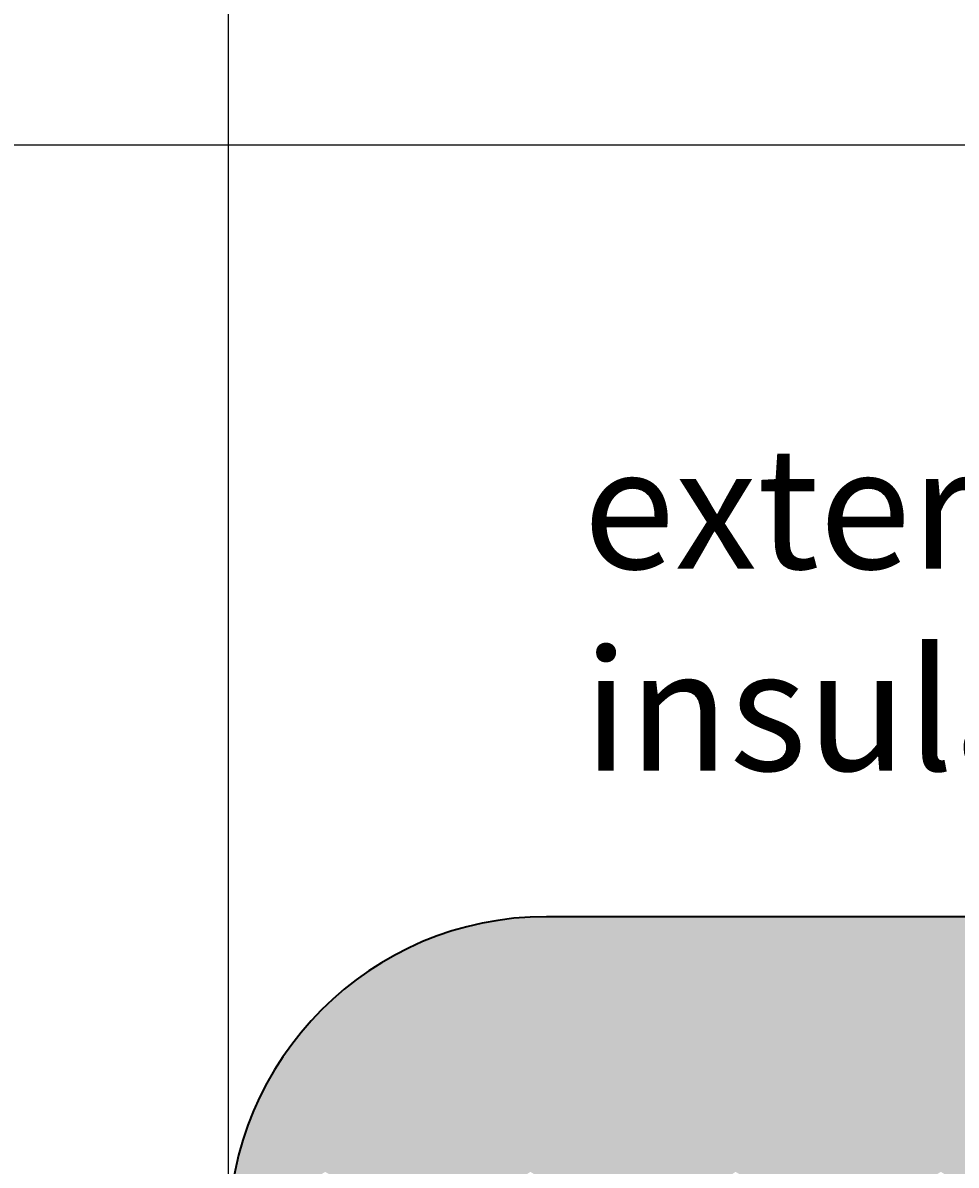
# Model space of a CAD drawing. Units: inches. Extents: x -1 to 292, y -3 to 199.
# Tile 12 of 52: x 45 to 68, y 101 to 130. Entities that reach past the tile are written whole.
import ezdxf

# ---------------------------------------------------------------- set-up
doc = ezdxf.new("R2010")
doc.units = ezdxf.units.IN
doc.header["$MEASUREMENT"] = 0
for name, color, linetype, lineweight in [('M-ANNO-TEXT', 3, 'Continuous', 25), ('M-DIMS', 2, 'Continuous', 18), ('M-EQPM', 7, 'Continuous', 35), ('M-PATT', 8, 'Continuous', 13)]:
    doc.layers.add(name, color=color, linetype=linetype, lineweight=lineweight)
doc.styles.get("Standard").update_dxf_attribs({"font": 'arial.ttf'})
doc.dimstyles.get("Standard").update_dxf_attribs({"dimtxt": 0.18, "dimasz": 0.18, "dimexe": 0.18, "dimexo": 0.0625, "dimgap": 0.09, "dimtad": 0, "dimtih": 1, "dimtoh": 1, "dimdec": 4, "dimzin": 0, "dimdsep": 46, "dimtxsty": 'Standard', "dimcen": 0.09, "dimadec": 0, "dimazin": 0, "dimtfac": 1, "dimtdec": 4, "dimtofl": 0, "dimtmove": 0, "dimatfit": 3, "dimfxl": 1, "dimtolj": 1, "dimtzin": 0, "dimarcsym": 0})

# ---------------------------------------------------------------- blocks, each defined once
blk = doc.blocks.new('*D8')
at = {"layer": 'Defpoints', "color": 0, "transparency": 16777216}
for p in [(-0.662, 126.765), (111.488, 126.765), (69.013, 25.514)]:
    blk.add_point(p, dxfattribs=at)
at = {"layer": 'M-DIMS', "color": 0, "lineweight": -2, "transparency": 16777216}
for p, q in [((111.426, 126.765), (-0.842, 126.765)), ((-0.662, 126.585), (-0.662, 76.321)), ((-0.662, 25.694), (-0.662, 75.958)), ((68.951, 25.514), (-0.842, 25.514))]:
    blk.add_line(p, q, dxfattribs=at)
at = {"layer": 'M-DIMS', "color": 0, "transparency": 16777216}
for points in [[(-0.692, 126.585), (-0.632, 126.585), (-0.662, 126.765)], [(-0.692, 25.694), (-0.632, 25.694), (-0.662, 25.514)]]:
    blk.add_solid(points, dxfattribs=at)
at = {"layer": 'M-DIMS', "color": 0, "transparency": 16777216, "insert": (-0.662, 76.14), "char_height": 0.18, "attachment_point": 5}
blk.add_mtext('\\A1;101.25', dxfattribs=at)
blk = doc.blocks.new('*D9')
at = {"layer": 'Defpoints', "color": 0, "transparency": 16777216}
for p in [(177.053, 174.363), (49.924, 99.774), (177.053, 99.774)]:
    blk.add_point(p, dxfattribs=at)
at = {"layer": 'M-DIMS', "color": 0, "lineweight": -2, "transparency": 16777216}
for p, q in [((49.924, 99.836), (49.924, 174.543)), ((50.104, 174.363), (113.033, 174.363)), ((176.873, 174.363), (113.943, 174.363)), ((177.053, 99.836), (177.053, 174.543))]:
    blk.add_line(p, q, dxfattribs=at)
at = {"layer": 'M-DIMS', "color": 0, "transparency": 16777216}
for points in [[(50.104, 174.393), (50.104, 174.333), (49.924, 174.363)], [(176.873, 174.393), (176.873, 174.333), (177.053, 174.363)]]:
    blk.add_solid(points, dxfattribs=at)
at = {"layer": 'M-DIMS', "color": 0, "transparency": 16777216, "insert": (113.488, 174.363), "char_height": 0.18, "attachment_point": 5}
blk.add_mtext('\\A1;127.13', dxfattribs=at)

msp = doc.modelspace()

# ---------------------------------------------------------------- hatches: boundary and pattern name
at = {"layer": 'M-PATT'}
h = msp.add_hatch(color=256, dxfattribs=at)
h.set_gradient(color1=(237, 31, 36), color2=(242, 113, 114), tint=1, name='CYLINDER')
h.paths.add_polyline_path([(106.0735, 105.9941), (106.0735, 106.9941), (108.0603, 106.9941), (107.8488, 107.6501), (57.8007, 107.6501, 0.4142136), (49.9241, 99.7735), (52.3176, 101.3278), (55.0097, 99.7735), (57.4032, 101.3278), (60.0953, 99.7735), (62.4888, 101.3278), (65.1809, 99.7735), (67.5744, 101.3278), (70.2665, 99.7735), (72.66, 101.3278), (75.3521, 99.7735), (77.7456, 101.3278), (80.4377, 99.7735), (82.8312, 101.3278), (85.5233, 99.7735), (87.9168, 101.3278), (90.6089, 99.7735), (93.0024, 101.3278), (95.6945, 99.7735), (98.088, 101.3278), (100.7801, 99.7735), (103.1736, 101.3278), (105.8657, 99.7735), (108.2592, 101.3278), (110.9513, 99.7735), (113.3448, 101.3278), (116.0369, 99.7735), (118.4304, 101.3278), (121.1225, 99.7735), (123.516, 101.3278), (126.2082, 99.7735), (128.6016, 101.3278), (131.2938, 99.7735), (133.6872, 101.3278), (136.3794, 99.7735), (138.7728, 101.3278), (141.465, 99.7735), (143.8584, 101.3278), (146.5506, 99.7735), (148.944, 101.3278), (151.6362, 99.7735), (154.0296, 101.3278), (156.7218, 99.7735), (159.1152, 101.3278), (160.6222, 100.4578), (160.6222, 107.6501), (115.4883, 107.6501), (115.4883, 106.9941), (120.9032, 106.9941), (120.9032, 105.9941), (120.9032, 103.3981), (106.0735, 103.3981)])
h.paths.add_polyline_path([(169.176, 107.6501), (162.1623, 107.6501), (162.1623, 100.004), (164.2008, 101.3278), (166.893, 99.7735), (169.2864, 101.3278), (171.9786, 99.7735), (174.372, 101.3278), (177.0526, 99.7802, 0.4139642)])
h.paths.add_polyline_path([(111.4883, 107.6501), (107.8488, 107.6501), (108.0603, 106.9941), (111.4883, 106.9941)], flags=17)
h.paths.add_polyline_path([(61.6788, 91.897), (57.8007, 91.897, -0.1099266), (54.4604, 92.6403), (43.2011, 92.6403), (23.9502, 84.4688), (23.9502, 58.376), (43.2011, 47.2615), (50.9409, 47.2615, -0.2705926), (57.8007, 51.2672), (61.6788, 51.2672)])
h.paths.add_polyline_path([(73.6788, 91.897), (70.6788, 91.897), (70.6788, 51.2672), (73.6788, 51.2672)])
h.paths.add_polyline_path([(79.6788, 91.897), (76.6788, 91.897), (76.6788, 51.2672), (79.6788, 51.2672)])
h.paths.add_polyline_path([(67.6788, 91.897), (64.6788, 91.897), (64.6788, 51.2672), (67.6788, 51.2672)])
h.paths.add_polyline_path([(101.6788, 91.897), (82.6788, 91.897), (82.6788, 51.2672), (101.6788, 51.2672)])
h.paths.add_polyline_path([(107.6788, 91.897), (104.6788, 91.897), (104.6788, 51.2672), (107.6788, 51.2672)])
h.paths.add_polyline_path([(113.6788, 91.897), (110.6788, 91.897), (110.6788, 51.2672), (113.6788, 51.2672)])
h.paths.add_polyline_path([(119.6788, 91.897), (116.6788, 91.897), (116.6788, 51.2672), (119.6788, 51.2672)])
h.paths.add_polyline_path([(141.6788, 91.897), (122.6788, 91.897), (122.6788, 51.2672), (141.6788, 51.2672)])
h.paths.add_polyline_path([(147.6788, 91.897), (144.6788, 91.897), (144.6788, 51.2672), (147.6788, 51.2672)])
h.paths.add_polyline_path([(153.6788, 91.897), (150.6788, 91.897), (150.6788, 51.2672), (153.6788, 51.2672)])
h.paths.add_polyline_path([(159.6788, 91.897), (156.6788, 91.897), (156.6788, 51.2672), (159.6788, 51.2672)])
h.paths.add_polyline_path([(179.5897, 92.6403), (172.5163, 92.6403, -0.1099266), (169.176, 91.897), (162.6788, 91.897), (162.6788, 51.2672), (169.176, 51.2672, -0.2705926), (176.0358, 47.2615), (179.5897, 47.2615)])
h.paths.add_polyline_path([(203.0265, 84.4688), (183.7755, 92.6403), (181.5897, 92.6403), (181.5897, 47.2615), (183.7755, 47.2615), (203.0265, 58.376)])
h.paths.add_polyline_path([(184.4188, 61.52), (200.7224, 61.52), (200.7224, 77.7532), (184.4188, 77.7532)], flags=24)

# ---------------------------------------------------------------- linework, layer by layer
at = {"layer": 'M-EQPM'}
msp.add_lwpolyline([(110.9873, 107.6501), (57.8007, 107.6501, 1), (57.8007, 91.897), (61.6788, 91.897)], format="xyb", dxfattribs=at)
msp.add_lwpolyline([(111.4883, 107.6501), (57.8007, 107.6501)], dxfattribs=at)

# ---------------------------------------------------------------- texts
at = {"layer": 'M-ANNO-TEXT', "insert": (58.713, 119.2686), "char_height": 3, "attachment_point": 1}
msp.add_mtext_dynamic_manual_height_columns('external \\Pinsulation', width=47.899539, gutter_width=1, heights=[0], dxfattribs=at)

# ---------------------------------------------------------------- dimensions: what is measured, and where the dimension line sits
at = {"layer": 'M-DIMS'}
dim = msp.add_linear_dim(base=(177.0526, 174.3627), p1=(49.9241, 99.7735), p2=(177.0526, 99.7735), dimstyle='Standard', override={"dimdec": 2, "dimlfac": 1, "dimrnd": 0, "dimzin": 0, "dimdsep": 46, "dimlunit": 2}, dxfattribs=at)
dim.commit()
dim.dimension.update_dxf_attribs({"geometry": '*D9', "text_midpoint": (113.4883, 174.3627)})
dim = msp.add_linear_dim(base=(-0.6625, 126.765), p1=(69.013, 25.5141), p2=(111.4883, 126.765), angle=90, dimstyle='Standard', override={"dimdec": 2, "dimlfac": 1, "dimrnd": 0, "dimzin": 0, "dimdsep": 46, "dimlunit": 2}, dxfattribs=at)
dim.commit()
dim.dimension.update_dxf_attribs({"geometry": '*D8', "text_midpoint": (-0.6625, 76.1396)})

doc.saveas('drawing.dxf')
